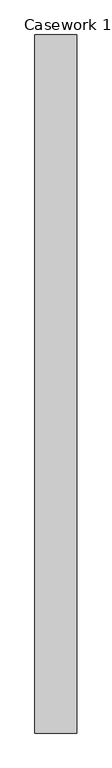
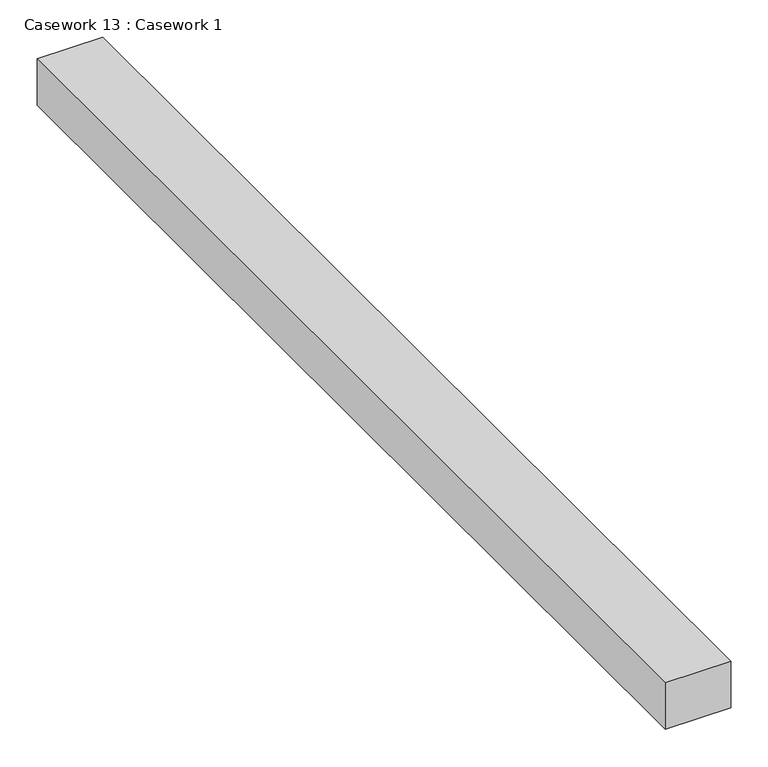
"""IFC4 building model written with IfcOpenShell, lengths in millimetres: furniture geometry, Casework 13 : Casework 1."""

from ifc_helpers import new_model, si_unit, frame, origin, place, context, project, spatial, polyline, outline, extrude, source, transform, mapped, element, save


def casework_13_casework_1_b548bcc5(model_context):
    return source(origin(), model_context, "Body", "SweptSolid", [
        extrude(outline(polyline([(6004.9559589, 14787.9496924), (6004.9559589, 13098.8496924), (5903.3559589, 13098.8496924), (5903.3559589, 14787.9496924), (6004.9559589, 14787.9496924)])), frame((0.0, 0.0, 3581.4), z_axis=(0.0, 0.0, 1.0), x_axis=(1.0, 0.0, 0.0)), (0.0, 0.0, 1.0), 76.2),
    ])


if __name__ == "__main__":
    model = new_model("IFC4")
    model_context = context("Model", 3, world=origin())
    ifc_project = project(units=[si_unit("LENGTHUNIT", "METRE", prefix="MILLI")], contexts=[model_context])
    site = spatial("IfcSite", under=ifc_project)
    building = spatial("IfcBuilding", under=site)
    placement = place(None, origin())
    casework_13_casework_1_shape = casework_13_casework_1_b548bcc5(model_context)
    element("IfcFurniture", 1, ObjectType="Casework 13 : Casework 1", at=placement, inside=building, context=model_context, shape_type="MappedRepresentation", body=[
        mapped(casework_13_casework_1_shape, transform((0.0, 0.0, 0.0), x_axis=(1.0, 0.0, 0.0), y_axis=(0.0, 1.0, 0.0), z_axis=(0.0, 0.0, 1.0))),
    ])
    save(model, "model.ifc")

# Revit data of these elements
# Element 1 (IfcFurniture, "Casework 13 : Casework 1")
#   Materials on its faces: "Clad - White"
# Materials
#   "Clad - White": class "Wood", colour RGB 242 242 238, transparency 0, Cost = 0
